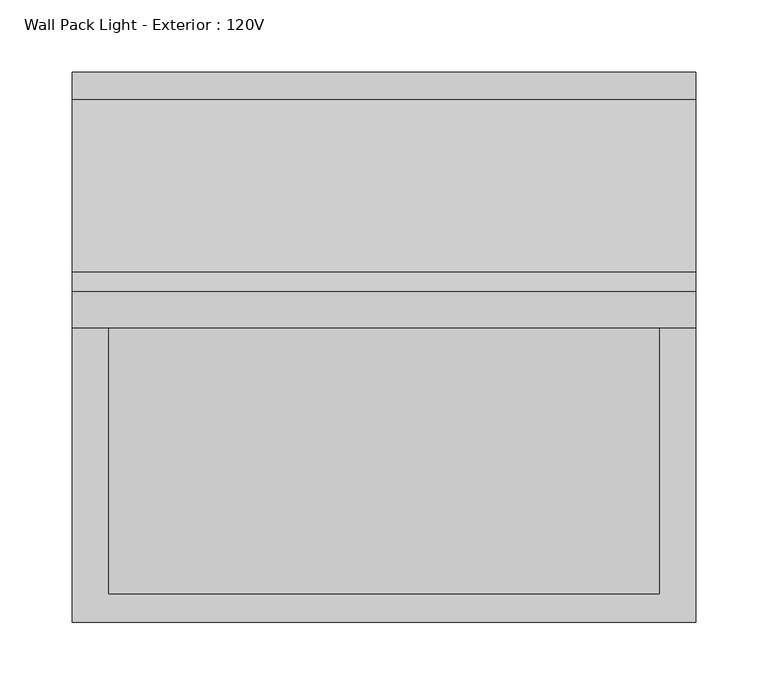
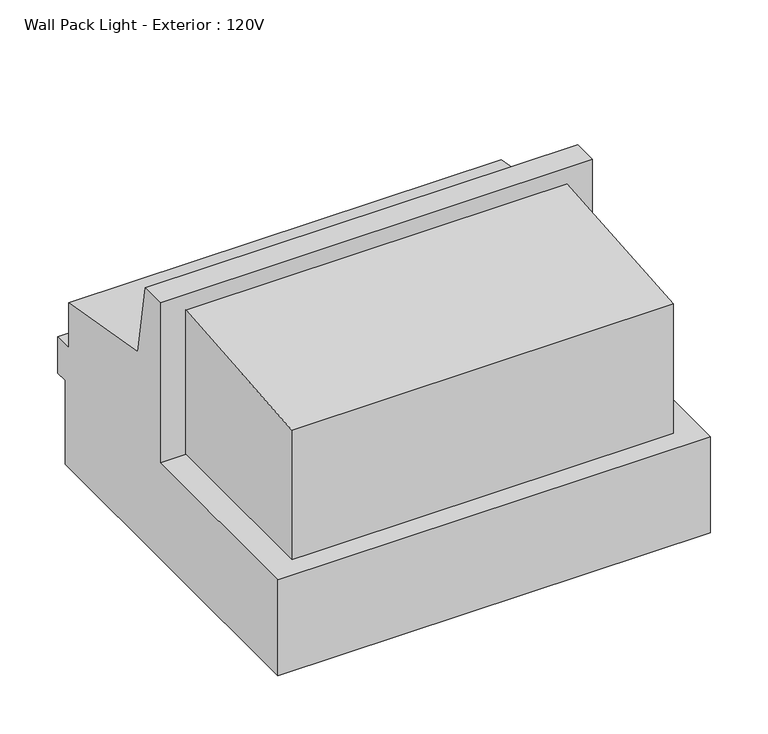
"""IFC4 building model written with IfcOpenShell, lengths in millimetres: light fixture geometry, Wall Pack Light - Exterior : 120V."""

from ifc_helpers import new_model, si_unit, frame, origin, place, context, project, spatial, polyline, outline, extrude, source, transform, mapped, element, save


def wall_pack_light_exterior_120v_ab60a804(model_context):
    return source(origin(), model_context, "Body", "SweptSolid", [
        extrude(outline(polyline([(184.15, 0.0), (-184.15, 0.0), (-184.15, 101.6), (19.84375, 101.6), (19.84375, 270.66875), (45.24375, 270.66875), (58.7375, 195.2625), (177.8, 174.625), (177.8, 127.0), (196.85, 127.0), (196.85, 88.9), (184.15, 88.9), (184.15, 0.0)])), frame((-215.9, 0.0, 0.0), z_axis=(1.0, 0.0, 0.0), x_axis=(0.0, 1.0, 0.0)), (0.0, 0.0, 1.0), 431.8),
        extrude(outline(polyline([(19.84375, 101.6), (-164.30625, 101.6), (-164.30625, 238.8195312), (19.84375, 254.0), (19.84375, 101.6)])), frame((-190.5, 0.0, 0.0), z_axis=(1.0, 0.0, 0.0), x_axis=(0.0, 1.0, 0.0)), (0.0, 0.0, 1.0), 381.0),
    ])


if __name__ == "__main__":
    model = new_model("IFC4")
    model_context = context("Model", 3, world=origin())
    ifc_project = project(units=[si_unit("LENGTHUNIT", "METRE", prefix="MILLI")], contexts=[model_context])
    site = spatial("IfcSite", under=ifc_project)
    building = spatial("IfcBuilding", under=site)
    placement = place(None, origin())
    wall_pack_light_exterior_120v_shape = wall_pack_light_exterior_120v_ab60a804(model_context)
    element("IfcLightFixture", 1, ObjectType="Wall Pack Light - Exterior : 120V", at=placement, inside=building, context=model_context, shape_type="MappedRepresentation", body=[
        mapped(wall_pack_light_exterior_120v_shape, transform((0.0, 0.0, 0.0), x_axis=(1.0, 0.0, 0.0), y_axis=(0.0, 1.0, 0.0), z_axis=(0.0, 0.0, 1.0))),
    ])
    save(model, "model.ifc")

# Revit data of these elements
# Type "Wall Pack Light - Exterior : 120V"
#   Photometric Web File = "WPE1MH.IES"
#   Wattage = 70 W
#   built-in parameter 1150110 = 1 (stored number, unit not read)
#   built-in parameter 1150109 = 1 (stored number, unit not read)
#   built-in parameter 1150113 = 1 (stored number, unit not read)
#   Tilt Angle = -90.00°
#   Lumens = 5499.9 lm
#   built-in parameter 1114217 = 1 (stored number, unit not read)
#   built-in parameter 1150115 = 1 (stored number, unit not read)
#   built-in parameter 1150105 = 437.668 (stored number, unit not read)
#   built-in parameter 1150112 = 1 (stored number, unit not read)
#   built-in parameter 1150114 = 1 (stored number, unit not read)
#   built-in parameter 1150107 = 4000 (stored number, unit not read)
#   built-in parameter 1150106 = 4.37668 (stored number, unit not read)
#   built-in parameter 1150104 = 7.29939 (stored number, unit not read)
#   Ballast Voltage = 120 V
#   Default Elevation = 9' - 0"
#   built-in parameter 1114218 = 1 (stored number, unit not read)
#   built-in parameter 1150133 = 10 (stored number, unit not read)
#   Apparent Load = 70 VA
#   built-in parameter 1150134 = 12
#   built-in parameter 1150137 = 1
#   Color Filter = 16777215
#   Ballast Number of Poles = 1
#   built-in parameter 1140040 [instance default] = 1
#   Wall Mount Material = Metal - Paint Finish - Dark Grey, Matte
#   Shade Material = Glass
#   Load Classification = Lighting - Exterior
#   Dimming Lamp Color Temperature Shift = (empty or 0)
# Element 1 (IfcLightFixture, "Wall Pack Light - Exterior : 120V")
#   Materials on its faces: "Metal - Paint Finish - Dark Grey, Matte", "Glass"
# Materials
#   "Metal - Paint Finish - Dark Grey, Matte": class "Paint", colour RGB 98 98 98, transparency 0
#   "Glass": class "Glass", colour RGB 0 128 192, transparency 0.75, Description = "Soda Lime Glass", Cost = 0
